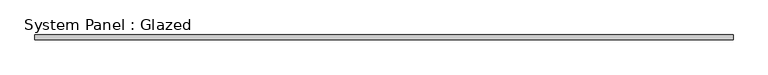
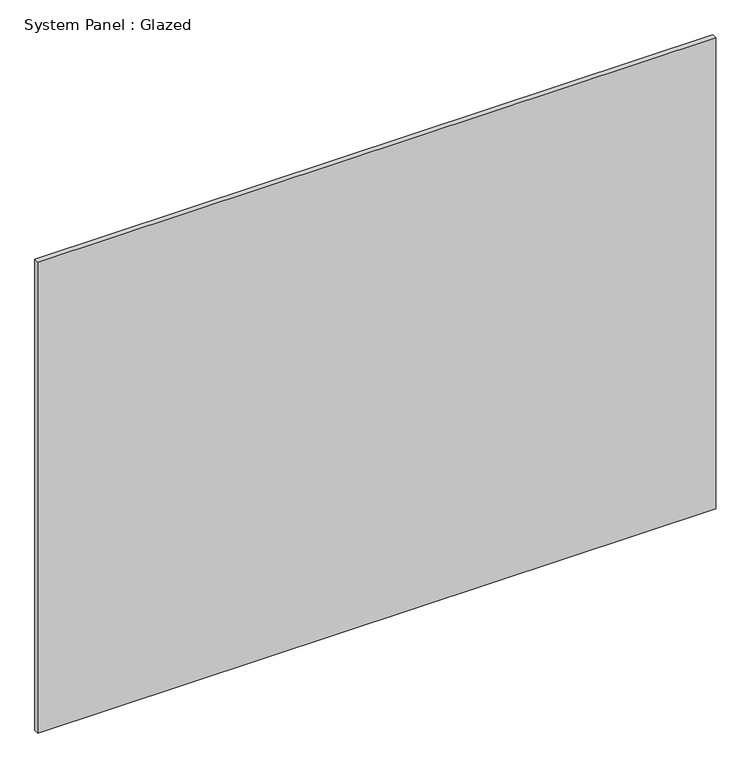
"""IFC4 building model written with IfcOpenShell, lengths in millimetres: plate geometry, System Panel : Glazed."""

from ifc_helpers import new_model, si_unit, origin, origin_with_axes, place, context, project, spatial, polyline, outline, extrude, source, transform, mapped, element, save


def system_panel_glazed_4346f86e(model_context):
    return source(origin(), model_context, "Body", "SweptSolid", [
        extrude(outline(polyline([(1781.175, 19.05), (-1781.175, 19.05), (-1781.175, 44.45), (1781.175, 44.45), (1781.175, 19.05)])), origin_with_axes(), (0.0, 0.0, 1.0), 2616.2),
    ])


if __name__ == "__main__":
    model = new_model("IFC4")
    model_context = context("Model", 3, world=origin())
    ifc_project = project(units=[si_unit("LENGTHUNIT", "METRE", prefix="MILLI")], contexts=[model_context])
    site = spatial("IfcSite", under=ifc_project)
    building = spatial("IfcBuilding", under=site)
    placement = place(None, origin())
    system_panel_glazed_shape = system_panel_glazed_4346f86e(model_context)
    element("IfcPlate", 1, ObjectType="System Panel : Glazed", at=placement, inside=building, context=model_context, shape_type="MappedRepresentation", body=[
        mapped(system_panel_glazed_shape, transform((0.0, 0.0, 0.0), x_axis=(1.0, 0.0, 0.0), y_axis=(0.0, 1.0, 0.0), z_axis=(0.0, 0.0, 1.0))),
    ])
    save(model, "model.ifc")

# Revit data of these elements
# Type "System Panel : Glazed"
#   Construction Type Id = "GSP4R"
#   Analytic Construction = "1/8 in Pilkington single glazing"
#   Visual Light Transmittance = 0.9
#   Solar Heat Gain Coefficient = 0.86
#   Heat Transfer Coefficient (U) = 1.18115 BTU/(h·ft²·°F)
# Element 1 (IfcPlate, "System Panel : Glazed")
#   Materials on its faces: "Glass"
# Materials
#   "Glass": class "Glass", colour RGB 0 128 192, transparency 0.75, Description = "Soda Lime Glass", Cost = 0
